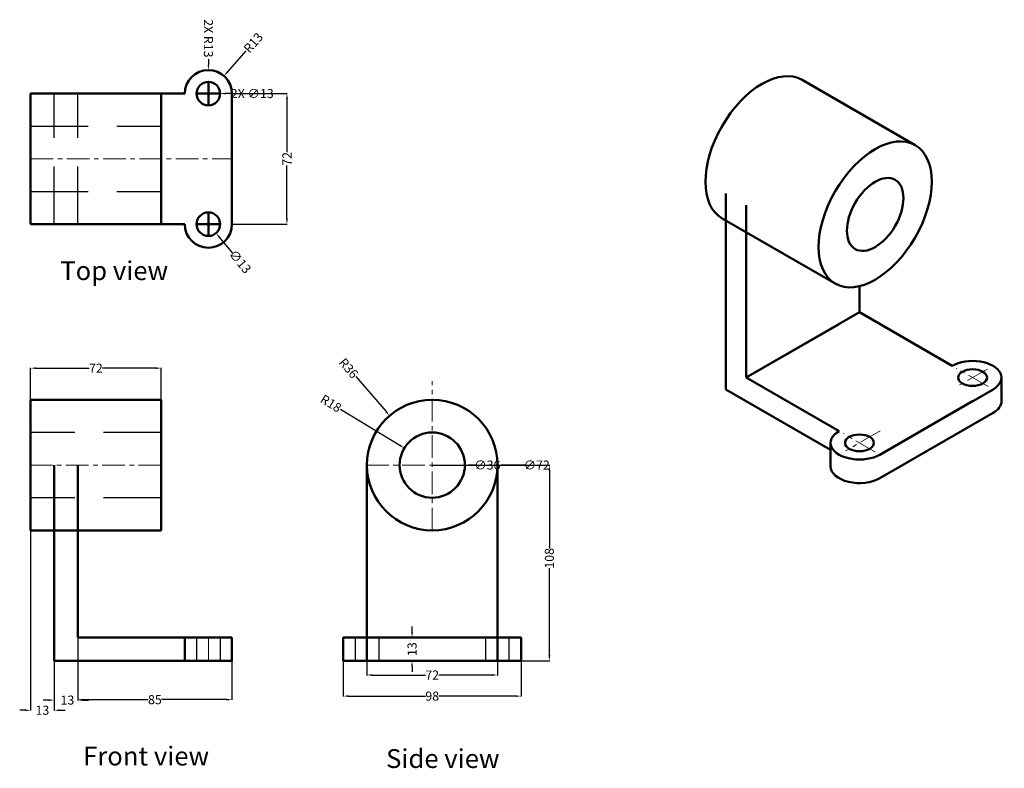
# Model space of a CAD drawing. Units: inches. Extents: x 66 to 609, y -14 to 399.
import ezdxf

# ---------------------------------------------------------------- set-up
doc = ezdxf.new("R2010")
doc.units = ezdxf.units.IN
doc.header["$MEASUREMENT"] = 0
doc.linetypes.add('CENTER', pattern=[2, 1.25, -0.25, 0.25, -0.25])
doc.linetypes.add('HIDDEN', pattern=[9.525, 6.35, -3.175])
for name, color, linetype, lineweight in [('M-CNTR', 4, 'CENTER', 18), ('M-DIMS', 2, 'Continuous', 25), ('M-HIDN', 1, 'HIDDEN', 25), ('M-OUTL', 7, 'Continuous', 50), ('M-TEXT', 3, 'Continuous', 25)]:
    doc.layers.add(name, color=color, linetype=linetype, lineweight=lineweight)
doc.styles.get("Standard").update_dxf_attribs({"font": 'arial.ttf'})
doc.dimstyles.get("Standard").update_dxf_attribs({"dimtxt": 5, "dimasz": 3, "dimexe": 0.18, "dimexo": 0.0625, "dimgap": 0.09, "dimtad": 0, "dimdec": 0, "dimzin": 0, "dimdsep": 46, "dimtxsty": 'Standard', "dimcen": 0.09, "dimadec": 0, "dimazin": 0, "dimtfac": 1, "dimtdec": 0, "dimtofl": 0, "dimtmove": 0, "dimatfit": 3, "dimfxl": 1, "dimtolj": 1, "dimtzin": 0, "dimarcsym": 0})

# ---------------------------------------------------------------- blocks, each defined once
blk = doc.blocks.new('*D1')
at = {"layer": 'Defpoints', "color": 0, "transparency": 16777216}
for p in [(293.24, 153.33), (357.8, 153.33), (293.24, 45.33)]:
    blk.add_point(p, dxfattribs=at)
at = {"layer": 'M-DIMS', "color": 0, "lineweight": -2, "transparency": 16777216}
for p, q in [((293.31, 153.33), (357.98, 153.33)), ((357.8, 150.33), (357.8, 107.3)), ((357.8, 48.33), (357.8, 96.54)), ((293.31, 45.33), (357.98, 45.33))]:
    blk.add_line(p, q, dxfattribs=at)
at = {"layer": 'M-DIMS', "color": 0, "transparency": 16777216}
for points in [[(357.3, 150.33), (358.3, 150.33), (357.8, 153.33)], [(357.3, 48.33), (358.3, 48.33), (357.8, 45.33)]]:
    blk.add_solid(points, dxfattribs=at)
at = {"layer": 'M-DIMS', "color": 0, "transparency": 16777216, "insert": (357.8, 101.92), "char_height": 5, "attachment_point": 5, "rotation": 90}
blk.add_mtext('\\A1;108', dxfattribs=at)
blk = doc.blocks.new('*D2')
at = {"layer": 'Defpoints', "color": 0, "transparency": 16777216}
for p in [(143.88, 206.78), (71.88, 189.33), (143.88, 189.33)]:
    blk.add_point(p, dxfattribs=at)
at = {"layer": 'M-DIMS', "color": 0, "lineweight": -2, "transparency": 16777216}
for p, q in [((71.88, 189.4), (71.88, 206.96)), ((74.88, 206.78), (104.25, 206.78)), ((140.88, 206.78), (111.5, 206.78)), ((143.88, 189.4), (143.88, 206.96))]:
    blk.add_line(p, q, dxfattribs=at)
at = {"layer": 'M-DIMS', "color": 0, "transparency": 16777216}
for points in [[(74.88, 207.28), (74.88, 206.28), (71.88, 206.78)], [(140.88, 207.28), (140.88, 206.28), (143.88, 206.78)]]:
    blk.add_solid(points, dxfattribs=at)
at = {"layer": 'M-DIMS', "color": 0, "transparency": 16777216, "insert": (107.88, 206.78), "char_height": 5, "attachment_point": 5}
blk.add_mtext('\\A1;72', dxfattribs=at)
blk = doc.blocks.new('*D3')
at = {"layer": 'Defpoints', "color": 0, "transparency": 16777216}
for p in [(97.88, 58.33), (84.88, 45.33), (97.88, 23.73)]:
    blk.add_point(p, dxfattribs=at)
at = {"layer": 'M-DIMS', "color": 0, "lineweight": -2, "transparency": 16777216}
for p, q in [((97.88, 58.27), (97.88, 23.55)), ((84.88, 45.27), (84.88, 23.55)), ((81.88, 23.73), (78.88, 23.73)), ((100.88, 23.73), (103.88, 23.73))]:
    blk.add_line(p, q, dxfattribs=at)
at = {"layer": 'M-DIMS', "color": 0, "transparency": 16777216}
for points in [[(81.88, 24.23), (81.88, 23.23), (84.88, 23.73)], [(100.88, 24.23), (100.88, 23.23), (97.88, 23.73)]]:
    blk.add_solid(points, dxfattribs=at)
at = {"layer": 'M-DIMS', "color": 0, "transparency": 16777216, "insert": (92.2, 23.73), "char_height": 5, "attachment_point": 5}
blk.add_mtext('\\A1;13', dxfattribs=at)
blk = doc.blocks.new('*D4')
at = {"layer": 'Defpoints', "color": 0, "transparency": 16777216}
for p in [(244.24, 45.33), (342.24, 45.33), (342.24, 25.93)]:
    blk.add_point(p, dxfattribs=at)
at = {"layer": 'M-DIMS', "color": 0, "lineweight": -2, "transparency": 16777216}
for p, q in [((244.24, 45.27), (244.24, 25.75)), ((342.24, 45.27), (342.24, 25.75)), ((247.24, 25.93), (289.57, 25.93)), ((339.24, 25.93), (296.92, 25.93))]:
    blk.add_line(p, q, dxfattribs=at)
at = {"layer": 'M-DIMS', "color": 0, "transparency": 16777216}
for points in [[(247.24, 26.43), (247.24, 25.43), (244.24, 25.93)], [(339.24, 26.43), (339.24, 25.43), (342.24, 25.93)]]:
    blk.add_solid(points, dxfattribs=at)
at = {"layer": 'M-DIMS', "color": 0, "transparency": 16777216, "insert": (293.24, 25.93), "char_height": 5, "attachment_point": 5}
blk.add_mtext('\\A1;98', dxfattribs=at)
blk = doc.blocks.new('*D5')
at = {"layer": 'Defpoints', "color": 0, "transparency": 16777216}
for p in [(257.24, 45.33), (329.24, 45.33), (329.24, 37.55)]:
    blk.add_point(p, dxfattribs=at)
at = {"layer": 'M-DIMS', "color": 0, "lineweight": -2, "transparency": 16777216}
for p, q in [((257.24, 45.27), (257.24, 37.37)), ((329.24, 45.27), (329.24, 37.37)), ((260.24, 37.55), (289.62, 37.55)), ((326.24, 37.55), (296.87, 37.55))]:
    blk.add_line(p, q, dxfattribs=at)
at = {"layer": 'M-DIMS', "color": 0, "transparency": 16777216}
for points in [[(260.24, 38.05), (260.24, 37.05), (257.24, 37.55)], [(326.24, 38.05), (326.24, 37.05), (329.24, 37.55)]]:
    blk.add_solid(points, dxfattribs=at)
at = {"layer": 'M-DIMS', "color": 0, "transparency": 16777216, "insert": (293.24, 37.55), "char_height": 5, "attachment_point": 5}
blk.add_mtext('\\A1;72', dxfattribs=at)
blk = doc.blocks.new('*D6')
at = {"layer": 'Defpoints', "color": 0, "transparency": 16777216}
for p in [(269.74, 180.6), (293.24, 153.33)]:
    blk.add_point(p, dxfattribs=at)
at = {"layer": 'M-DIMS', "color": 0, "lineweight": -2, "transparency": 16777216}
for p, q in [((251.13, 202.18), (267.78, 182.87)), ((293.15, 153.33), (293.33, 153.33)), ((293.24, 153.24), (293.24, 153.42))]:
    blk.add_line(p, q, dxfattribs=at)
at = {"layer": 'M-DIMS', "color": 0, "transparency": 16777216}
blk.add_solid([(268.16, 183.2), (267.4, 182.55), (269.74, 180.6)], dxfattribs=at)
at = {"layer": 'M-DIMS', "color": 0, "transparency": 16777216, "insert": (247.17, 206.77), "char_height": 5, "attachment_point": 5, "rotation": 310.7683}
blk.add_mtext('\\A1;R36', dxfattribs=at)
blk = doc.blocks.new('*D7')
at = {"layer": 'Defpoints', "color": 0, "transparency": 16777216}
for p in [(277.87, 162.7), (293.24, 153.33)]:
    blk.add_point(p, dxfattribs=at)
at = {"layer": 'M-DIMS', "color": 0, "lineweight": -2, "transparency": 16777216}
for p, q in [((242.63, 184.18), (275.31, 164.26)), ((293.15, 153.33), (293.33, 153.33)), ((293.24, 153.24), (293.24, 153.42))]:
    blk.add_line(p, q, dxfattribs=at)
at = {"layer": 'M-DIMS', "color": 0, "transparency": 16777216}
blk.add_solid([(275.57, 164.69), (275.05, 163.84), (277.87, 162.7)], dxfattribs=at)
at = {"layer": 'M-DIMS', "color": 0, "transparency": 16777216, "insert": (237.45, 187.34), "char_height": 5, "attachment_point": 5, "rotation": 328.6402}
blk.add_mtext('\\A1;R18', dxfattribs=at)
blk = doc.blocks.new('*D8')
at = {"layer": 'Defpoints', "color": 0, "transparency": 16777216}
for p in [(277.14, 58.33), (277.14, 45.33), (282.12, 45.33)]:
    blk.add_point(p, dxfattribs=at)
at = {"layer": 'M-DIMS', "color": 0, "lineweight": -2, "transparency": 16777216}
for p, q in [((282.12, 61.33), (282.12, 64.33)), ((277.2, 58.33), (282.3, 58.33)), ((277.2, 45.33), (282.3, 45.33)), ((282.12, 42.33), (282.12, 39.33))]:
    blk.add_line(p, q, dxfattribs=at)
at = {"layer": 'M-DIMS', "color": 0, "transparency": 16777216}
for points in [[(281.62, 61.33), (282.62, 61.33), (282.12, 58.33)], [(281.62, 42.33), (282.62, 42.33), (282.12, 45.33)]]:
    blk.add_solid(points, dxfattribs=at)
at = {"layer": 'M-DIMS', "color": 0, "transparency": 16777216, "insert": (282.12, 51.83), "char_height": 5, "attachment_point": 5, "rotation": 90}
blk.add_mtext('\\A1;13', dxfattribs=at)
blk = doc.blocks.new('*D9')
at = {"layer": 'Defpoints', "color": 0, "transparency": 16777216}
for p in [(97.88, 58.33), (182.88, 58.33), (182.88, 23.98)]:
    blk.add_point(p, dxfattribs=at)
at = {"layer": 'M-DIMS', "color": 0, "lineweight": -2, "transparency": 16777216}
for p, q in [((97.88, 58.27), (97.88, 23.8)), ((182.88, 58.27), (182.88, 23.8)), ((100.88, 23.98), (136.68, 23.98)), ((179.88, 23.98), (144.07, 23.98))]:
    blk.add_line(p, q, dxfattribs=at)
at = {"layer": 'M-DIMS', "color": 0, "transparency": 16777216}
for points in [[(100.88, 24.48), (100.88, 23.48), (97.88, 23.98)], [(179.88, 24.48), (179.88, 23.48), (182.88, 23.98)]]:
    blk.add_solid(points, dxfattribs=at)
at = {"layer": 'M-DIMS', "color": 0, "transparency": 16777216, "insert": (140.38, 23.98), "char_height": 5, "attachment_point": 5}
blk.add_mtext('\\A1;85', dxfattribs=at)
blk = doc.blocks.new('*D10')
at = {"layer": 'Defpoints', "color": 0, "transparency": 16777216}
for p in [(182.88, 358.18), (213.19, 358.18), (182.88, 286.18)]:
    blk.add_point(p, dxfattribs=at)
at = {"layer": 'M-DIMS', "color": 0, "lineweight": -2, "transparency": 16777216}
for p, q in [((182.94, 358.18), (213.37, 358.18)), ((213.19, 355.18), (213.19, 325.8)), ((213.19, 289.18), (213.19, 318.55)), ((182.94, 286.18), (213.37, 286.18))]:
    blk.add_line(p, q, dxfattribs=at)
at = {"layer": 'M-DIMS', "color": 0, "transparency": 16777216}
for points in [[(212.69, 355.18), (213.69, 355.18), (213.19, 358.18)], [(212.69, 289.18), (213.69, 289.18), (213.19, 286.18)]]:
    blk.add_solid(points, dxfattribs=at)
at = {"layer": 'M-DIMS', "color": 0, "transparency": 16777216, "insert": (213.19, 322.18), "char_height": 5, "attachment_point": 5, "rotation": 90}
blk.add_mtext('\\A1;72', dxfattribs=at)
blk = doc.blocks.new('*D11')
at = {"layer": 'Defpoints', "color": 0, "transparency": 16777216}
for p in [(178.47, 367.93), (169.88, 358.18)]:
    blk.add_point(p, dxfattribs=at)
at = {"layer": 'M-DIMS', "color": 0, "lineweight": -2, "transparency": 16777216}
for p, q in [((190.6, 381.7), (180.45, 370.18)), ((169.79, 358.18), (169.97, 358.18)), ((169.88, 358.09), (169.88, 358.27))]:
    blk.add_line(p, q, dxfattribs=at)
at = {"layer": 'M-DIMS', "color": 0, "transparency": 16777216}
blk.add_solid([(180.08, 370.51), (180.83, 369.85), (178.47, 367.93)], dxfattribs=at)
at = {"layer": 'M-DIMS', "color": 0, "transparency": 16777216, "insert": (194.61, 386.25), "char_height": 5, "attachment_point": 5, "rotation": 48.6156}
blk.add_mtext('\\A1;R13', dxfattribs=at)
blk = doc.blocks.new('*D12')
at = {"layer": 'Defpoints', "color": 0, "transparency": 16777216}
for p in [(165.67, 291.14), (174.08, 281.22)]:
    blk.add_point(p, dxfattribs=at)
at = {"layer": 'M-DIMS', "color": 0, "lineweight": -2, "transparency": 16777216}
for p, q in [((169.79, 286.18), (169.97, 286.18)), ((169.88, 286.09), (169.88, 286.27)), ((183.24, 270.42), (176.02, 278.93))]:
    blk.add_line(p, q, dxfattribs=at)
at = {"layer": 'M-DIMS', "color": 0, "transparency": 16777216}
blk.add_solid([(176.4, 279.26), (175.64, 278.61), (174.08, 281.22)], dxfattribs=at)
at = {"layer": 'M-DIMS', "color": 0, "transparency": 16777216, "insert": (187.38, 265.55), "char_height": 5, "attachment_point": 5, "rotation": 310.3021}
blk.add_mtext('\\A1;∅13', dxfattribs=at)
blk = doc.blocks.new('HOLE-MOUNT')
for p, q in [((6.5, 0), (6.5, 13)), ((0, 6.5), (13, 6.5))]:
    blk.add_line(p, q)
blk.add_circle((6.5, 6.5), 6.5)
blk = doc.blocks.new('*D14')
at = {"layer": 'Defpoints', "color": 0, "transparency": 16777216}
for p in [(71.877049, 117.334807), (84.877049, 45.334807), (84.877049, 18.134807)]:
    blk.add_point(p, dxfattribs=at)
at = {"layer": 'M-DIMS', "color": 0, "lineweight": -2, "transparency": 16777216}
for p, q in [((71.877049, 117.272307), (71.877049, 17.954807)), ((84.877049, 45.272307), (84.877049, 17.954807)), ((68.877049, 18.134807), (65.877049, 18.134807)), ((87.877049, 18.134807), (90.877049, 18.134807))]:
    blk.add_line(p, q, dxfattribs=at)
at = {"layer": 'M-DIMS', "color": 0, "transparency": 16777216}
for points in [[(68.877049, 18.634807), (68.877049, 17.634807), (71.877049, 18.134807)], [(87.877049, 18.634807), (87.877049, 17.634807), (84.877049, 18.134807)]]:
    blk.add_solid(points, dxfattribs=at)
at = {"layer": 'M-DIMS', "color": 0, "transparency": 16777216, "insert": (78.377049, 18.134807), "char_height": 5, "attachment_point": 5}
blk.add_mtext('\\A1;13', dxfattribs=at)
blk = doc.blocks.new('*D15')
at = {"layer": 'Defpoints', "color": 0, "transparency": 16777216}
for p in [(257.24, 153.33), (329.24, 153.34)]:
    blk.add_point(p, dxfattribs=at)
at = {"layer": 'M-DIMS', "color": 0, "lineweight": -2, "transparency": 16777216}
for p, q in [((293.15, 153.33), (293.33, 153.33)), ((293.24, 153.24), (293.24, 153.42)), ((344.48, 153.34), (332.24, 153.34))]:
    blk.add_line(p, q, dxfattribs=at)
at = {"layer": 'M-DIMS', "color": 0, "transparency": 16777216}
blk.add_solid([(332.24, 153.84), (332.24, 152.84), (329.24, 153.34)], dxfattribs=at)
at = {"layer": 'M-DIMS', "color": 0, "transparency": 16777216, "insert": (350.84, 153.34), "char_height": 5, "attachment_point": 5, "rotation": 0.0003}
blk.add_mtext('\\A1;∅72', dxfattribs=at)
blk = doc.blocks.new('*D16')
at = {"layer": 'Defpoints', "color": 0, "transparency": 16777216}
for p in [(275.24, 153.33), (311.24, 153.34)]:
    blk.add_point(p, dxfattribs=at)
at = {"layer": 'M-DIMS', "color": 0, "lineweight": -2, "transparency": 16777216}
for p, q in [((293.15, 153.33), (293.33, 153.33)), ((293.24, 153.24), (293.24, 153.42)), ((317.24, 153.34), (314.24, 153.34))]:
    blk.add_line(p, q, dxfattribs=at)
at = {"layer": 'M-DIMS', "color": 0, "transparency": 16777216}
blk.add_solid([(314.24, 153.84), (314.24, 152.84), (311.24, 153.34)], dxfattribs=at)
at = {"layer": 'M-DIMS', "color": 0, "transparency": 16777216, "insert": (323.63, 153.34), "char_height": 5, "attachment_point": 5, "rotation": 0.0006}
blk.add_mtext('\\A1;∅36', dxfattribs=at)
blk = doc.blocks.new('*D17')
at = {"layer": 'Defpoints', "color": 0, "transparency": 16777216}
for p in [(169.88, 371.18), (169.88, 358.18)]:
    blk.add_point(p, dxfattribs=at)
at = {"layer": 'M-DIMS', "color": 0, "lineweight": -2, "transparency": 16777216}
for p, q in [((169.88, 377.18), (169.88, 374.18)), ((169.79, 358.18), (169.97, 358.18)), ((169.88, 358.09), (169.88, 358.27))]:
    blk.add_line(p, q, dxfattribs=at)
at = {"layer": 'M-DIMS', "color": 0, "transparency": 16777216}
blk.add_solid([(170.38, 374.18), (169.38, 374.18), (169.88, 371.18)], dxfattribs=at)
at = {"layer": 'M-DIMS', "color": 0, "transparency": 16777216, "insert": (169.88, 388.66), "char_height": 5, "attachment_point": 5, "rotation": 270.0002}
blk.add_mtext('\\A1;2X R13', dxfattribs=at)
blk = doc.blocks.new('*D18')
at = {"layer": 'Defpoints', "color": 0, "transparency": 16777216}
for p in [(163.38, 358.17), (176.38, 358.19)]:
    blk.add_point(p, dxfattribs=at)
at = {"layer": 'M-DIMS', "color": 0, "lineweight": -2, "transparency": 16777216}
for p, q in [((169.79, 358.18), (169.97, 358.18)), ((169.88, 358.09), (169.88, 358.27)), ((182.38, 358.19), (179.38, 358.19))]:
    blk.add_line(p, q, dxfattribs=at)
at = {"layer": 'M-DIMS', "color": 0, "transparency": 16777216}
blk.add_solid([(179.38, 358.69), (179.38, 357.69), (176.38, 358.19)], dxfattribs=at)
at = {"layer": 'M-DIMS', "color": 0, "transparency": 16777216, "insert": (194.05, 358.2), "char_height": 5, "attachment_point": 5, "rotation": 0.056}
blk.add_mtext('\\A1;2X ∅13', dxfattribs=at)

msp = doc.modelspace()

# ---------------------------------------------------------------- linework, layer by layer
at = {"layer": 'M-CNTR', "ltscale": 10}
for p, q in [((71.88, 322.18), (182.88, 322.18)), ((599.64, 196.67), (582.17, 206.7)), ((599.09, 206.18), (582.12, 196.5)), ((293.24, 117.33), (293.24, 199.62)), ((537.52, 160.48), (519.75, 170.74)), ((540.15, 172.17), (521.05, 161.14)), ((143.88, 153.33), (71.88, 153.33)), ((329.24, 153.33), (257.24, 153.33)), ((169.88, 58.33), (169.88, 45.33))]:
    msp.add_line(p, q, dxfattribs=at)
at = {"layer": 'M-HIDN', "ltscale": 5}
for p, q in [((84.88, 286.18), (84.88, 358.18)), ((97.88, 286.18), (97.88, 358.18)), ((71.88, 340.18), (143.88, 340.18)), ((71.88, 304.18), (143.88, 304.18)), ((143.88, 171.33), (71.88, 171.33)), ((143.88, 135.33), (71.88, 135.33)), ((163.38, 58.33), (163.38, 45.33)), ((176.38, 58.33), (176.38, 45.33)), ((250.74, 58.33), (250.74, 45.33)), ((263.74, 58.33), (263.74, 45.33)), ((322.74, 45.33), (322.74, 58.33)), ((335.74, 45.33), (335.74, 58.33))]:
    msp.add_line(p, q, dxfattribs=at)
at = {"layer": 'M-OUTL'}
for p, q in [((559.42, 329.75), (497.06, 365.75)), ((71.88, 358.18), (156.88, 358.18)), ((71.88, 286.18), (71.88, 358.18)), ((143.88, 286.18), (143.88, 358.18)), ((182.88, 286.18), (182.88, 358.18)), ((455.1, 303.07), (455.1, 195.07)), ((466.36, 296.57), (466.36, 201.57)), ((515.33, 253.38), (452.97, 289.38)), ((71.88, 286.18), (156.88, 286.18)), ((528.71, 251.98), (528.71, 237.57)), ((528.71, 237.57), (466.36, 201.57)), ((579.81, 208.07), (528.71, 237.57)), ((466.36, 201.57), (517.45, 231.07)), ((517.45, 172.07), (466.36, 201.57)), ((606.99, 201.57), (606.99, 188.57)), ((455.1, 195.07), (512.79, 161.76)), ((602.32, 195.07), (539.97, 159.07)), ((143.88, 189.33), (71.88, 189.33)), ((71.88, 153.33), (71.88, 189.33)), ((143.88, 117.33), (143.88, 189.33)), ((539.97, 159.07), (591.07, 188.57)), ((602.32, 182.07), (539.97, 146.07)), ((512.79, 165.57), (512.79, 152.57)), ((71.88, 117.33), (71.88, 153.33)), ((84.88, 153.33), (84.88, 45.33)), ((97.88, 153.33), (97.88, 58.33)), ((257.24, 153.33), (257.24, 45.33)), ((329.24, 45.33), (329.24, 153.33)), ((143.88, 117.33), (71.88, 117.33)), ((97.88, 58.33), (182.88, 58.33)), ((156.88, 58.33), (156.88, 45.33)), ((182.88, 58.33), (182.88, 45.33)), ((244.24, 58.33), (342.24, 58.33)), ((244.24, 58.33), (244.24, 45.33)), ((342.24, 45.33), (342.24, 58.33)), ((84.88, 45.33), (182.88, 45.33)), ((244.24, 45.33), (342.24, 45.33))]:
    msp.add_line(p, q, dxfattribs=at)
for radius in [36, 18]:
    msp.add_circle((293.24, 153.33), radius, dxfattribs=at)
for centre, start, end in [((169.88, 358.18), 0, 180), ((169.88, 286.18), 180, 0)]:
    msp.add_arc(centre, 13, start, end, dxfattribs=at)
for centre, major_axis, start_param, end_param in [((475.02, 327.57), (-22.05, -38.18), 3.141593, 6.283185), ((591.07, 201.57), (-15.92, 0), 2.356194, 5.497787), ((591.07, 188.57), (-15.92, 0), 2.356194, 3.141593), ((528.71, 165.57), (-15.92, 0), 5.497787, 8.63938), ((528.71, 152.57), (-15.92, 0), 6.283185, 8.63938)]:
    msp.add_ellipse(centre, major_axis=major_axis, ratio=0.57735, start_param=start_param, end_param=end_param, dxfattribs=at)
for centre, major_axis in [((537.37, 291.57), (-22.05, -38.18)), ((537.37, 291.57), (-11.02, -19.09)), ((591.07, 201.57), (-7.96, 0)), ((528.71, 165.57), (-7.96, 0))]:
    msp.add_ellipse(centre, major_axis=major_axis, ratio=0.57735, dxfattribs=at)

# ---------------------------------------------------------------- block references
for p in [(163.38, 351.68), (163.38, 279.68)]:
    msp.add_blockref('HOLE-MOUNT', p, dxfattribs=at)

# ---------------------------------------------------------------- texts
at = {"layer": 'M-TEXT', "char_height": 10.364, "attachment_point": 1}
for s, insert in [('Top view', (88.26, 265.71)), ('Front view', (100.85, -1.96)), ('Side view', (267.82, -3.34))]:
    msp.add_mtext_dynamic_manual_height_columns(s, width=101.9316, gutter_width=1.04, heights=[0], dxfattribs=dict(at, insert=insert))

# ---------------------------------------------------------------- dimensions: what is measured, and where the dimension line sits
at = {"layer": 'M-DIMS'}
dim = msp.add_radius_dim(center=(169.88, 358.18), mpoint=(169.88, 371.18), text='2X <>', dimstyle='Standard', override={"dimdec": 0, "dimlfac": 1, "dimrnd": 0, "dimzin": 0, "dimdsep": 46, "dimlunit": 2}, dxfattribs=at)
dim.commit()
dim.dimension.update_dxf_attribs({"geometry": '*D17', "text_midpoint": (169.88, 388.66)})
for center, mpoint, picture, middle in [((169.88, 358.18), (178.47, 367.93), '*D11', (194.61, 386.25)), ((293.24, 153.33), (269.74, 180.6), '*D6', (247.17, 206.77)), ((293.24, 153.33), (277.87, 162.7), '*D7', (237.45, 187.34))]:
    dim = msp.add_radius_dim(center=center, mpoint=mpoint, dimstyle='Standard', override={"dimclrd": 0, "dimclre": 0, "dimclrt": 0}, dxfattribs=at)
    dim.commit()
    dim.dimension.update_dxf_attribs({"geometry": picture, "text_midpoint": middle, "dimtype": 164})
dim = msp.add_diameter_dim_2p(p1=(163.38, 358.17), p2=(176.38, 358.19), text='2X <>', dimstyle='Standard', override={"dimdec": 0, "dimlfac": 1, "dimrnd": 0, "dimzin": 0, "dimdsep": 46, "dimlunit": 2}, dxfattribs=at)
dim.commit()
dim.dimension.update_dxf_attribs({"geometry": '*D18', "text_midpoint": (194.05, 358.2)})
for base, p1, p2, picture, middle in [((213.19, 358.18), (182.88, 286.18), (182.88, 358.18), '*D10', (213.19, 322.18)), ((282.12, 45.33), (277.14, 58.33), (277.14, 45.33), '*D8', (282.12, 51.83))]:
    dim = msp.add_linear_dim(base=base, p1=p1, p2=p2, angle=90, dimstyle='Standard', override={"dimclrd": 0, "dimclre": 0, "dimclrt": 0}, dxfattribs=at)
    dim.commit()
    dim.dimension.update_dxf_attribs({"geometry": picture, "text_midpoint": middle})
for p1, p2, override, picture, middle in [((165.67, 291.14), (174.08, 281.22), {"dimclrd": 0, "dimclre": 0, "dimclrt": 0}, '*D12', (187.38, 265.55)), ((257.24, 153.33), (329.24, 153.34), {"dimdec": 0, "dimlfac": 1, "dimrnd": 0, "dimzin": 0, "dimdsep": 46, "dimlunit": 2}, '*D15', (350.84, 153.34))]:
    dim = msp.add_diameter_dim_2p(p1=p1, p2=p2, dimstyle='Standard', override=override, dxfattribs=at)
    dim.commit()
    dim.dimension.update_dxf_attribs({"geometry": picture, "text_midpoint": middle, "dimtype": 163})
for base, p1, p2, override, picture, middle in [((143.88, 206.78), (71.88, 189.33), (143.88, 189.33), {"dimclrd": 0, "dimclre": 0, "dimclrt": 0}, '*D2', (107.88, 206.78)), ((84.88, 18.13), (71.88, 117.33), (84.88, 45.33), {"dimdec": 0, "dimlfac": 1, "dimrnd": 0, "dimzin": 0, "dimdsep": 46, "dimlunit": 2}, '*D14', (78.38, 18.13)), ((182.88, 23.98), (97.88, 58.33), (182.88, 58.33), {"dimclrd": 0, "dimclre": 0, "dimclrt": 0}, '*D9', (140.38, 23.98)), ((342.24, 25.93), (244.24, 45.33), (342.24, 45.33), {"dimclrd": 0, "dimclre": 0, "dimclrt": 0}, '*D4', (293.24, 25.93)), ((329.24, 37.55), (257.24, 45.33), (329.24, 45.33), {"dimclrd": 0, "dimclre": 0, "dimclrt": 0}, '*D5', (293.24, 37.55))]:
    dim = msp.add_linear_dim(base=base, p1=p1, p2=p2, dimstyle='Standard', override=override, dxfattribs=at)
    dim.commit()
    dim.dimension.update_dxf_attribs({"geometry": picture, "text_midpoint": middle})
dim = msp.add_diameter_dim_2p(p1=(275.24, 153.33), p2=(311.24, 153.34), dimstyle='Standard', override={"dimdec": 0, "dimlfac": 1, "dimrnd": 0, "dimzin": 0, "dimdsep": 46, "dimlunit": 2}, dxfattribs=at)
dim.commit()
dim.dimension.update_dxf_attribs({"geometry": '*D16', "text_midpoint": (323.63, 153.34)})
dim = msp.add_linear_dim(base=(357.8, 153.33), p1=(293.24, 45.33), p2=(293.24, 153.33), angle=90, dimstyle='Standard', override={"dimclrd": 0, "dimclre": 0, "dimclrt": 0}, dxfattribs=at)
dim.commit()
dim.dimension.update_dxf_attribs({"geometry": '*D1', "text_midpoint": (357.8, 101.92), "dimtype": 160})
dim = msp.add_linear_dim(base=(97.88, 23.73), p1=(84.88, 45.33), p2=(97.88, 58.33), dimstyle='Standard', override={"dimclrd": 0, "dimclre": 0, "dimclrt": 0}, dxfattribs=at)
dim.commit()
dim.dimension.update_dxf_attribs({"geometry": '*D3', "text_midpoint": (92.2, 23.73), "dimtype": 160})

doc.saveas('drawing.dxf')
